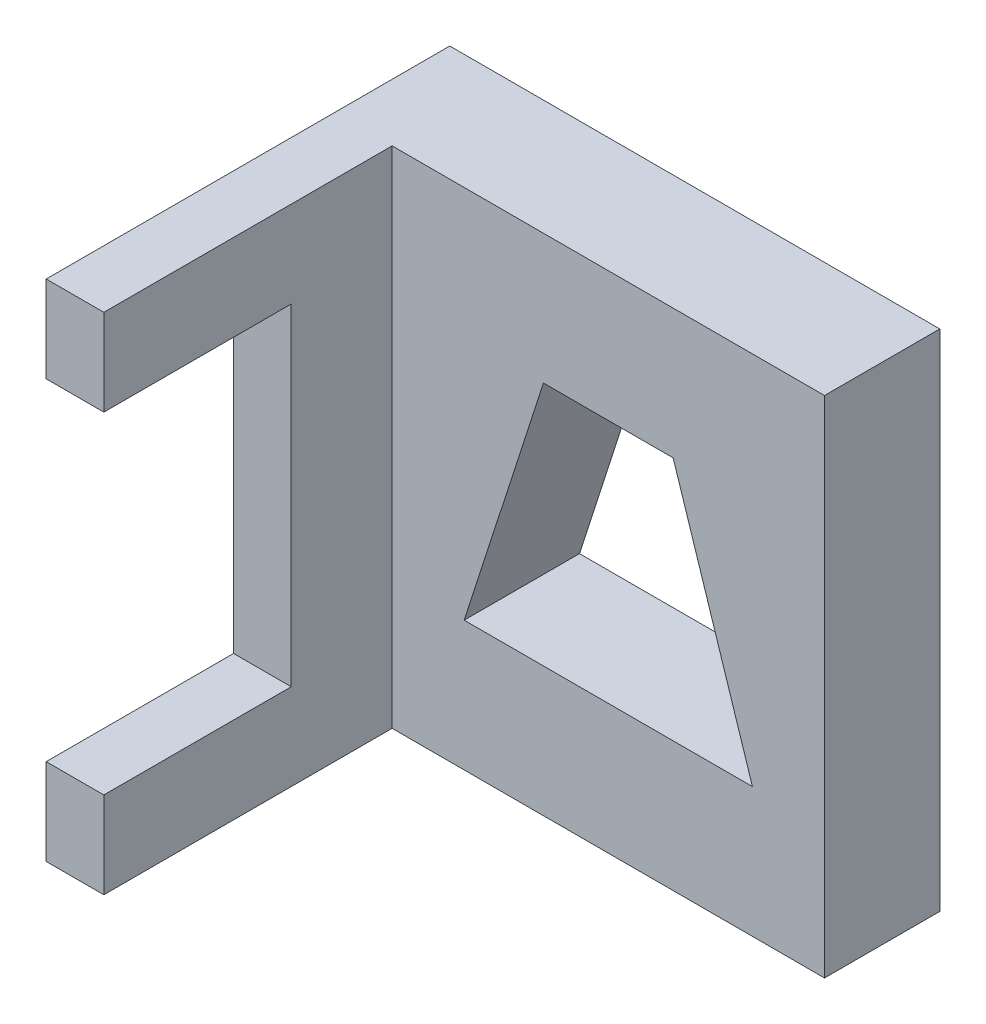
ISO-10303-21;
HEADER;
FILE_DESCRIPTION(('STEP AP214'),'2;1');
FILE_NAME('part.step','',(''),(''),'','','');
FILE_SCHEMA(('AUTOMOTIVE_DESIGN { 1 0 10303 214 1 1 1 1 }'));
ENDSEC;
DATA;
#1=APPLICATION_CONTEXT('core data for automotive mechanical design processes');
#2=APPLICATION_PROTOCOL_DEFINITION('international standard','automotive_design',2000,#1);
#3=PRODUCT_CONTEXT('',#1,'mechanical');
#4=PRODUCT('Part','Part','',(#3));
#5=PRODUCT_RELATED_PRODUCT_CATEGORY('part','',(#4));
#6=PRODUCT_DEFINITION_FORMATION('','',#4);
#7=PRODUCT_DEFINITION_CONTEXT('part definition',#1,'design');
#8=PRODUCT_DEFINITION('design','',#6,#7);
#9=PRODUCT_DEFINITION_SHAPE('','',#8);
#10=(LENGTH_UNIT() NAMED_UNIT(*) SI_UNIT(.MILLI.,.METRE.));
#11=(NAMED_UNIT(*) PLANE_ANGLE_UNIT() SI_UNIT($,.RADIAN.));
#12=(NAMED_UNIT(*) SI_UNIT($,.STERADIAN.) SOLID_ANGLE_UNIT());
#13=UNCERTAINTY_MEASURE_WITH_UNIT(LENGTH_MEASURE(1.E-05),#10,'distance_accuracy_value','');
#14=(GEOMETRIC_REPRESENTATION_CONTEXT(3) GLOBAL_UNCERTAINTY_ASSIGNED_CONTEXT((#13)) GLOBAL_UNIT_ASSIGNED_CONTEXT((#10,
#11,#12)) REPRESENTATION_CONTEXT('',''));
#15=CARTESIAN_POINT('',(0.,0.,0.));
#16=DIRECTION('',(0.,0.,1.));
#17=DIRECTION('',(1.,0.,0.));
#18=AXIS2_PLACEMENT_3D('',#15,#16,#17);
#19=CARTESIAN_POINT('',(0.,0.,16.));
#20=DIRECTION('',(0.,0.,1.));
#21=DIRECTION('',(1.,0.,0.));
#22=AXIS2_PLACEMENT_3D('',#19,#20,#21);
#23=PLANE('',#22);
#24=DIRECTION('',(-0.307820285414663,0.951444518554411,0.));
#25=VECTOR('',#24,1.);
#26=CARTESIAN_POINT('',(47.,52.,16.));
#27=LINE('',#26,#25);
#28=CARTESIAN_POINT('',(58.,18.,16.));
#29=VERTEX_POINT('',#28);
#30=CARTESIAN_POINT('',(47.,52.,16.));
#31=VERTEX_POINT('',#30);
#32=EDGE_CURVE('E58',#29,#31,#27,.T.);
#33=ORIENTED_EDGE('',*,*,#32,.F.);
#34=DIRECTION('',(1.,0.,0.));
#35=VECTOR('',#34,1.);
#36=CARTESIAN_POINT('',(58.,18.,16.));
#37=LINE('',#36,#35);
#38=CARTESIAN_POINT('',(18.,18.,16.));
#39=VERTEX_POINT('',#38);
#40=EDGE_CURVE('E163',#39,#29,#37,.T.);
#41=ORIENTED_EDGE('',*,*,#40,.F.);
#42=DIRECTION('',(-0.307820285414662,-0.951444518554411,0.));
#43=VECTOR('',#42,1.);
#44=CARTESIAN_POINT('',(18.,18.,16.));
#45=LINE('',#44,#43);
#46=CARTESIAN_POINT('',(29.,52.,16.));
#47=VERTEX_POINT('',#46);
#48=EDGE_CURVE('E149',#47,#39,#45,.T.);
#49=ORIENTED_EDGE('',*,*,#48,.F.);
#50=DIRECTION('',(-1.,0.,0.));
#51=VECTOR('',#50,1.);
#52=CARTESIAN_POINT('',(29.,52.,16.));
#53=LINE('',#52,#51);
#54=EDGE_CURVE('E158',#31,#47,#53,.T.);
#55=ORIENTED_EDGE('',*,*,#54,.F.);
#56=EDGE_LOOP('',(#33,#41,#49,#55));
#57=FACE_BOUND('',#56,.T.);
#58=DIRECTION('',(-1.,0.,0.));
#59=VECTOR('',#58,1.);
#60=CARTESIAN_POINT('',(68.,70.,16.));
#61=LINE('',#60,#59);
#62=CARTESIAN_POINT('',(68.,70.,16.));
#63=VERTEX_POINT('',#62);
#64=CARTESIAN_POINT('',(8.,70.,16.));
#65=VERTEX_POINT('',#64);
#66=EDGE_CURVE('E226',#63,#65,#61,.T.);
#67=ORIENTED_EDGE('',*,*,#66,.T.);
#68=DIRECTION('',(0.,-1.,0.));
#69=VECTOR('',#68,1.);
#70=CARTESIAN_POINT('',(8.,0.,16.));
#71=LINE('',#70,#69);
#72=CARTESIAN_POINT('',(8.,0.,16.));
#73=VERTEX_POINT('',#72);
#74=EDGE_CURVE('E215',#65,#73,#71,.T.);
#75=ORIENTED_EDGE('',*,*,#74,.T.);
#76=DIRECTION('',(1.,0.,0.));
#77=VECTOR('',#76,1.);
#78=CARTESIAN_POINT('',(0.,0.,16.));
#79=LINE('',#78,#77);
#80=CARTESIAN_POINT('',(68.,0.,16.));
#81=VERTEX_POINT('',#80);
#82=EDGE_CURVE('E223',#73,#81,#79,.T.);
#83=ORIENTED_EDGE('',*,*,#82,.T.);
#84=DIRECTION('',(0.,1.,0.));
#85=VECTOR('',#84,1.);
#86=CARTESIAN_POINT('',(68.,0.,16.));
#87=LINE('',#86,#85);
#88=EDGE_CURVE('E229',#81,#63,#87,.T.);
#89=ORIENTED_EDGE('',*,*,#88,.T.);
#90=EDGE_LOOP('',(#67,#75,#83,#89));
#91=FACE_BOUND('',#90,.T.);
#92=ADVANCED_FACE('F44',(#57,#91),#23,.T.);
#93=CARTESIAN_POINT('',(0.,70.,16.));
#94=DIRECTION('',(1.,0.,0.));
#95=DIRECTION('',(0.,0.,-1.));
#96=AXIS2_PLACEMENT_3D('',#93,#94,#95);
#97=PLANE('',#96);
#98=DIRECTION('',(0.,-1.,0.));
#99=VECTOR('',#98,1.);
#100=CARTESIAN_POINT('',(0.,70.,0.));
#101=LINE('',#100,#99);
#102=CARTESIAN_POINT('',(0.,70.,0.));
#103=VERTEX_POINT('',#102);
#104=CARTESIAN_POINT('',(0.,0.,0.));
#105=VERTEX_POINT('',#104);
#106=EDGE_CURVE('E221',#103,#105,#101,.T.);
#107=ORIENTED_EDGE('',*,*,#106,.T.);
#108=DIRECTION('',(0.,0.,-1.));
#109=VECTOR('',#108,1.);
#110=CARTESIAN_POINT('',(0.,0.,16.));
#111=LINE('',#110,#109);
#112=CARTESIAN_POINT('',(0.,0.,56.));
#113=VERTEX_POINT('',#112);
#114=EDGE_CURVE('E249',#113,#105,#111,.T.);
#115=ORIENTED_EDGE('',*,*,#114,.F.);
#116=DIRECTION('',(0.,1.,0.));
#117=VECTOR('',#116,1.);
#118=CARTESIAN_POINT('',(0.,0.,56.));
#119=LINE('',#118,#117);
#120=CARTESIAN_POINT('',(0.,12.,56.));
#121=VERTEX_POINT('',#120);
#122=EDGE_CURVE('E173',#113,#121,#119,.T.);
#123=ORIENTED_EDGE('',*,*,#122,.T.);
#124=DIRECTION('',(0.,0.,-1.));
#125=VECTOR('',#124,1.);
#126=CARTESIAN_POINT('',(0.,12.,56.));
#127=LINE('',#126,#125);
#128=CARTESIAN_POINT('',(0.,12.,30.));
#129=VERTEX_POINT('',#128);
#130=EDGE_CURVE('E196',#121,#129,#127,.T.);
#131=ORIENTED_EDGE('',*,*,#130,.T.);
#132=DIRECTION('',(0.,1.,0.));
#133=VECTOR('',#132,1.);
#134=CARTESIAN_POINT('',(0.,12.,30.));
#135=LINE('',#134,#133);
#136=CARTESIAN_POINT('',(0.,58.,30.));
#137=VERTEX_POINT('',#136);
#138=EDGE_CURVE('E203',#129,#137,#135,.T.);
#139=ORIENTED_EDGE('',*,*,#138,.T.);
#140=DIRECTION('',(0.,0.,1.));
#141=VECTOR('',#140,1.);
#142=CARTESIAN_POINT('',(0.,58.,56.));
#143=LINE('',#142,#141);
#144=CARTESIAN_POINT('',(0.,58.,56.));
#145=VERTEX_POINT('',#144);
#146=EDGE_CURVE('E204',#137,#145,#143,.T.);
#147=ORIENTED_EDGE('',*,*,#146,.T.);
#148=DIRECTION('',(0.,1.,0.));
#149=VECTOR('',#148,1.);
#150=CARTESIAN_POINT('',(0.,70.,56.));
#151=LINE('',#150,#149);
#152=CARTESIAN_POINT('',(0.,70.,56.));
#153=VERTEX_POINT('',#152);
#154=EDGE_CURVE('E179',#145,#153,#151,.T.);
#155=ORIENTED_EDGE('',*,*,#154,.T.);
#156=DIRECTION('',(0.,0.,-1.));
#157=VECTOR('',#156,1.);
#158=CARTESIAN_POINT('',(0.,70.,16.));
#159=LINE('',#158,#157);
#160=EDGE_CURVE('E232',#153,#103,#159,.T.);
#161=ORIENTED_EDGE('',*,*,#160,.T.);
#162=EDGE_LOOP('',(#107,#115,#123,#131,#139,#147,#155,#161));
#163=FACE_BOUND('',#162,.T.);
#164=ADVANCED_FACE('F50',(#163),#97,.F.);
#165=CARTESIAN_POINT('',(0.,0.,16.));
#166=DIRECTION('',(0.,1.,0.));
#167=DIRECTION('',(0.,0.,1.));
#168=AXIS2_PLACEMENT_3D('',#165,#166,#167);
#169=PLANE('',#168);
#170=DIRECTION('',(1.,0.,0.));
#171=VECTOR('',#170,1.);
#172=CARTESIAN_POINT('',(0.,0.,0.));
#173=LINE('',#172,#171);
#174=CARTESIAN_POINT('',(68.,0.,0.));
#175=VERTEX_POINT('',#174);
#176=EDGE_CURVE('E235',#105,#175,#173,.T.);
#177=ORIENTED_EDGE('',*,*,#176,.T.);
#178=DIRECTION('',(0.,0.,-1.));
#179=VECTOR('',#178,1.);
#180=CARTESIAN_POINT('',(68.,0.,16.));
#181=LINE('',#180,#179);
#182=EDGE_CURVE('E241',#81,#175,#181,.T.);
#183=ORIENTED_EDGE('',*,*,#182,.F.);
#184=ORIENTED_EDGE('',*,*,#82,.F.);
#185=DIRECTION('',(0.,0.,1.));
#186=VECTOR('',#185,1.);
#187=CARTESIAN_POINT('',(8.,0.,0.));
#188=LINE('',#187,#186);
#189=CARTESIAN_POINT('',(8.,0.,56.));
#190=VERTEX_POINT('',#189);
#191=EDGE_CURVE('E177',#73,#190,#188,.T.);
#192=ORIENTED_EDGE('',*,*,#191,.T.);
#193=DIRECTION('',(-1.,0.,0.));
#194=VECTOR('',#193,1.);
#195=CARTESIAN_POINT('',(8.,0.,56.));
#196=LINE('',#195,#194);
#197=EDGE_CURVE('E195',#190,#113,#196,.T.);
#198=ORIENTED_EDGE('',*,*,#197,.T.);
#199=ORIENTED_EDGE('',*,*,#114,.T.);
#200=EDGE_LOOP('',(#177,#183,#184,#192,#198,#199));
#201=FACE_BOUND('',#200,.T.);
#202=ADVANCED_FACE('F278',(#201),#169,.F.);
#203=CARTESIAN_POINT('',(68.,0.,16.));
#204=DIRECTION('',(-1.,0.,0.));
#205=DIRECTION('',(0.,0.,1.));
#206=AXIS2_PLACEMENT_3D('',#203,#204,#205);
#207=PLANE('',#206);
#208=DIRECTION('',(0.,1.,0.));
#209=VECTOR('',#208,1.);
#210=CARTESIAN_POINT('',(68.,0.,0.));
#211=LINE('',#210,#209);
#212=CARTESIAN_POINT('',(68.,70.,0.));
#213=VERTEX_POINT('',#212);
#214=EDGE_CURVE('E240',#175,#213,#211,.T.);
#215=ORIENTED_EDGE('',*,*,#214,.T.);
#216=DIRECTION('',(0.,0.,-1.));
#217=VECTOR('',#216,1.);
#218=CARTESIAN_POINT('',(68.,70.,16.));
#219=LINE('',#218,#217);
#220=EDGE_CURVE('E244',#63,#213,#219,.T.);
#221=ORIENTED_EDGE('',*,*,#220,.F.);
#222=ORIENTED_EDGE('',*,*,#88,.F.);
#223=ORIENTED_EDGE('',*,*,#182,.T.);
#224=EDGE_LOOP('',(#215,#221,#222,#223));
#225=FACE_BOUND('',#224,.T.);
#226=ADVANCED_FACE('F290',(#225),#207,.F.);
#227=CARTESIAN_POINT('',(68.,70.,16.));
#228=DIRECTION('',(0.,-1.,0.));
#229=DIRECTION('',(0.,0.,-1.));
#230=AXIS2_PLACEMENT_3D('',#227,#228,#229);
#231=PLANE('',#230);
#232=ORIENTED_EDGE('',*,*,#160,.F.);
#233=DIRECTION('',(-1.,0.,0.));
#234=VECTOR('',#233,1.);
#235=CARTESIAN_POINT('',(8.,70.,56.));
#236=LINE('',#235,#234);
#237=CARTESIAN_POINT('',(8.,70.,56.));
#238=VERTEX_POINT('',#237);
#239=EDGE_CURVE('E207',#238,#153,#236,.T.);
#240=ORIENTED_EDGE('',*,*,#239,.F.);
#241=DIRECTION('',(0.,0.,-1.));
#242=VECTOR('',#241,1.);
#243=CARTESIAN_POINT('',(8.,70.,16.));
#244=LINE('',#243,#242);
#245=EDGE_CURVE('E175',#238,#65,#244,.T.);
#246=ORIENTED_EDGE('',*,*,#245,.T.);
#247=ORIENTED_EDGE('',*,*,#66,.F.);
#248=ORIENTED_EDGE('',*,*,#220,.T.);
#249=DIRECTION('',(-1.,0.,0.));
#250=VECTOR('',#249,1.);
#251=CARTESIAN_POINT('',(68.,70.,0.));
#252=LINE('',#251,#250);
#253=EDGE_CURVE('E227',#213,#103,#252,.T.);
#254=ORIENTED_EDGE('',*,*,#253,.T.);
#255=EDGE_LOOP('',(#232,#240,#246,#247,#248,#254));
#256=FACE_BOUND('',#255,.T.);
#257=ADVANCED_FACE('F287',(#256),#231,.F.);
#258=CARTESIAN_POINT('',(0.,0.,0.));
#259=DIRECTION('',(0.,0.,1.));
#260=DIRECTION('',(1.,0.,0.));
#261=AXIS2_PLACEMENT_3D('',#258,#259,#260);
#262=PLANE('',#261);
#263=DIRECTION('',(1.,0.,0.));
#264=VECTOR('',#263,1.);
#265=CARTESIAN_POINT('',(0.,18.,0.));
#266=LINE('',#265,#264);
#267=CARTESIAN_POINT('',(18.,18.,0.));
#268=VERTEX_POINT('',#267);
#269=CARTESIAN_POINT('',(58.,18.,0.));
#270=VERTEX_POINT('',#269);
#271=EDGE_CURVE('E52',#268,#270,#266,.T.);
#272=ORIENTED_EDGE('',*,*,#271,.T.);
#273=DIRECTION('',(-0.307820285414663,0.951444518554411,0.));
#274=VECTOR('',#273,1.);
#275=CARTESIAN_POINT('',(57.7760375880971,18.6922474549726,0.));
#276=LINE('',#275,#274);
#277=CARTESIAN_POINT('',(47.,52.,0.));
#278=VERTEX_POINT('',#277);
#279=EDGE_CURVE('E11',#270,#278,#276,.T.);
#280=ORIENTED_EDGE('',*,*,#279,.T.);
#281=DIRECTION('',(-1.,0.,0.));
#282=VECTOR('',#281,1.);
#283=CARTESIAN_POINT('',(0.,52.,0.));
#284=LINE('',#283,#282);
#285=CARTESIAN_POINT('',(29.,52.,0.));
#286=VERTEX_POINT('',#285);
#287=EDGE_CURVE('E253',#278,#286,#284,.T.);
#288=ORIENTED_EDGE('',*,*,#287,.T.);
#289=DIRECTION('',(-0.307820285414662,-0.951444518554412,0.));
#290=VECTOR('',#289,1.);
#291=CARTESIAN_POINT('',(11.0227094753328,-3.56617071260768,0.));
#292=LINE('',#291,#290);
#293=EDGE_CURVE('E155',#286,#268,#292,.T.);
#294=ORIENTED_EDGE('',*,*,#293,.T.);
#295=EDGE_LOOP('',(#272,#280,#288,#294));
#296=FACE_BOUND('',#295,.T.);
#297=ORIENTED_EDGE('',*,*,#106,.F.);
#298=ORIENTED_EDGE('',*,*,#253,.F.);
#299=ORIENTED_EDGE('',*,*,#214,.F.);
#300=ORIENTED_EDGE('',*,*,#176,.F.);
#301=EDGE_LOOP('',(#297,#298,#299,#300));
#302=FACE_BOUND('',#301,.T.);
#303=ADVANCED_FACE('F254',(#296,#302),#262,.F.);
#304=CARTESIAN_POINT('',(8.,70.,56.));
#305=DIRECTION('',(0.,0.,1.));
#306=DIRECTION('',(1.,0.,0.));
#307=AXIS2_PLACEMENT_3D('',#304,#305,#306);
#308=PLANE('',#307);
#309=ORIENTED_EDGE('',*,*,#154,.F.);
#310=DIRECTION('',(-1.,0.,0.));
#311=VECTOR('',#310,1.);
#312=CARTESIAN_POINT('',(8.,58.,56.));
#313=LINE('',#312,#311);
#314=CARTESIAN_POINT('',(8.,58.,56.));
#315=VERTEX_POINT('',#314);
#316=EDGE_CURVE('E213',#315,#145,#313,.T.);
#317=ORIENTED_EDGE('',*,*,#316,.F.);
#318=DIRECTION('',(0.,1.,0.));
#319=VECTOR('',#318,1.);
#320=CARTESIAN_POINT('',(8.,70.,56.));
#321=LINE('',#320,#319);
#322=EDGE_CURVE('E192',#315,#238,#321,.T.);
#323=ORIENTED_EDGE('',*,*,#322,.T.);
#324=ORIENTED_EDGE('',*,*,#239,.T.);
#325=EDGE_LOOP('',(#309,#317,#323,#324));
#326=FACE_BOUND('',#325,.T.);
#327=ADVANCED_FACE('F286',(#326),#308,.T.);
#328=CARTESIAN_POINT('',(8.,58.,56.));
#329=DIRECTION('',(0.,-1.,0.));
#330=DIRECTION('',(0.,0.,-1.));
#331=AXIS2_PLACEMENT_3D('',#328,#329,#330);
#332=PLANE('',#331);
#333=ORIENTED_EDGE('',*,*,#146,.F.);
#334=DIRECTION('',(-1.,0.,0.));
#335=VECTOR('',#334,1.);
#336=CARTESIAN_POINT('',(8.,58.,30.));
#337=LINE('',#336,#335);
#338=CARTESIAN_POINT('',(8.,58.,30.));
#339=VERTEX_POINT('',#338);
#340=EDGE_CURVE('E214',#339,#137,#337,.T.);
#341=ORIENTED_EDGE('',*,*,#340,.F.);
#342=DIRECTION('',(0.,0.,1.));
#343=VECTOR('',#342,1.);
#344=CARTESIAN_POINT('',(8.,58.,56.));
#345=LINE('',#344,#343);
#346=EDGE_CURVE('E190',#339,#315,#345,.T.);
#347=ORIENTED_EDGE('',*,*,#346,.T.);
#348=ORIENTED_EDGE('',*,*,#316,.T.);
#349=EDGE_LOOP('',(#333,#341,#347,#348));
#350=FACE_BOUND('',#349,.T.);
#351=ADVANCED_FACE('F330',(#350),#332,.T.);
#352=CARTESIAN_POINT('',(8.,12.,30.));
#353=DIRECTION('',(0.,0.,1.));
#354=DIRECTION('',(0.,-1.,0.));
#355=AXIS2_PLACEMENT_3D('',#352,#353,#354);
#356=PLANE('',#355);
#357=ORIENTED_EDGE('',*,*,#138,.F.);
#358=DIRECTION('',(-1.,0.,0.));
#359=VECTOR('',#358,1.);
#360=CARTESIAN_POINT('',(8.,12.,30.));
#361=LINE('',#360,#359);
#362=CARTESIAN_POINT('',(8.,12.,30.));
#363=VERTEX_POINT('',#362);
#364=EDGE_CURVE('E220',#363,#129,#361,.T.);
#365=ORIENTED_EDGE('',*,*,#364,.F.);
#366=DIRECTION('',(0.,1.,0.));
#367=VECTOR('',#366,1.);
#368=CARTESIAN_POINT('',(8.,12.,30.));
#369=LINE('',#368,#367);
#370=EDGE_CURVE('E188',#363,#339,#369,.T.);
#371=ORIENTED_EDGE('',*,*,#370,.T.);
#372=ORIENTED_EDGE('',*,*,#340,.T.);
#373=EDGE_LOOP('',(#357,#365,#371,#372));
#374=FACE_BOUND('',#373,.T.);
#375=ADVANCED_FACE('F324',(#374),#356,.T.);
#376=CARTESIAN_POINT('',(8.,12.,56.));
#377=DIRECTION('',(0.,1.,0.));
#378=DIRECTION('',(0.,0.,1.));
#379=AXIS2_PLACEMENT_3D('',#376,#377,#378);
#380=PLANE('',#379);
#381=ORIENTED_EDGE('',*,*,#130,.F.);
#382=DIRECTION('',(-1.,0.,0.));
#383=VECTOR('',#382,1.);
#384=CARTESIAN_POINT('',(8.,12.,56.));
#385=LINE('',#384,#383);
#386=CARTESIAN_POINT('',(8.,12.,56.));
#387=VERTEX_POINT('',#386);
#388=EDGE_CURVE('E218',#387,#121,#385,.T.);
#389=ORIENTED_EDGE('',*,*,#388,.F.);
#390=DIRECTION('',(0.,0.,-1.));
#391=VECTOR('',#390,1.);
#392=CARTESIAN_POINT('',(8.,12.,56.));
#393=LINE('',#392,#391);
#394=EDGE_CURVE('E181',#387,#363,#393,.T.);
#395=ORIENTED_EDGE('',*,*,#394,.T.);
#396=ORIENTED_EDGE('',*,*,#364,.T.);
#397=EDGE_LOOP('',(#381,#389,#395,#396));
#398=FACE_BOUND('',#397,.T.);
#399=ADVANCED_FACE('F325',(#398),#380,.T.);
#400=CARTESIAN_POINT('',(8.,0.,56.));
#401=DIRECTION('',(0.,0.,1.));
#402=DIRECTION('',(1.,0.,0.));
#403=AXIS2_PLACEMENT_3D('',#400,#401,#402);
#404=PLANE('',#403);
#405=ORIENTED_EDGE('',*,*,#122,.F.);
#406=ORIENTED_EDGE('',*,*,#197,.F.);
#407=DIRECTION('',(0.,1.,0.));
#408=VECTOR('',#407,1.);
#409=CARTESIAN_POINT('',(8.,0.,56.));
#410=LINE('',#409,#408);
#411=EDGE_CURVE('E180',#190,#387,#410,.T.);
#412=ORIENTED_EDGE('',*,*,#411,.T.);
#413=ORIENTED_EDGE('',*,*,#388,.T.);
#414=EDGE_LOOP('',(#405,#406,#412,#413));
#415=FACE_BOUND('',#414,.T.);
#416=ADVANCED_FACE('F269',(#415),#404,.T.);
#417=CARTESIAN_POINT('',(8.,0.,0.));
#418=DIRECTION('',(-1.,0.,0.));
#419=DIRECTION('',(0.,0.,1.));
#420=AXIS2_PLACEMENT_3D('',#417,#418,#419);
#421=PLANE('',#420);
#422=ORIENTED_EDGE('',*,*,#74,.F.);
#423=ORIENTED_EDGE('',*,*,#245,.F.);
#424=ORIENTED_EDGE('',*,*,#322,.F.);
#425=ORIENTED_EDGE('',*,*,#346,.F.);
#426=ORIENTED_EDGE('',*,*,#370,.F.);
#427=ORIENTED_EDGE('',*,*,#394,.F.);
#428=ORIENTED_EDGE('',*,*,#411,.F.);
#429=ORIENTED_EDGE('',*,*,#191,.F.);
#430=EDGE_LOOP('',(#422,#423,#424,#425,#426,#427,#428,#429));
#431=FACE_BOUND('',#430,.T.);
#432=ADVANCED_FACE('F265',(#431),#421,.F.);
#433=CARTESIAN_POINT('',(47.,52.,-2.));
#434=DIRECTION('',(0.951444518554411,0.307820285414662,0.));
#435=DIRECTION('',(-0.307820285414663,0.951444518554411,0.));
#436=AXIS2_PLACEMENT_3D('',#433,#434,#435);
#437=PLANE('',#436);
#438=DIRECTION('',(0.,0.,1.));
#439=VECTOR('',#438,1.);
#440=CARTESIAN_POINT('',(58.,18.,-2.));
#441=LINE('',#440,#439);
#442=EDGE_CURVE('E166',#270,#29,#441,.T.);
#443=ORIENTED_EDGE('',*,*,#442,.T.);
#444=ORIENTED_EDGE('',*,*,#32,.T.);
#445=DIRECTION('',(0.,0.,1.));
#446=VECTOR('',#445,1.);
#447=CARTESIAN_POINT('',(47.,52.,-2.));
#448=LINE('',#447,#446);
#449=EDGE_CURVE('E154',#278,#31,#448,.T.);
#450=ORIENTED_EDGE('',*,*,#449,.F.);
#451=ORIENTED_EDGE('',*,*,#279,.F.);
#452=EDGE_LOOP('',(#443,#444,#450,#451));
#453=FACE_BOUND('',#452,.T.);
#454=ADVANCED_FACE('F257',(#453),#437,.F.);
#455=CARTESIAN_POINT('',(58.,18.,-2.));
#456=DIRECTION('',(0.,-1.,0.));
#457=DIRECTION('',(0.,0.,-1.));
#458=AXIS2_PLACEMENT_3D('',#455,#456,#457);
#459=PLANE('',#458);
#460=DIRECTION('',(0.,0.,1.));
#461=VECTOR('',#460,1.);
#462=CARTESIAN_POINT('',(18.,18.,-2.));
#463=LINE('',#462,#461);
#464=EDGE_CURVE('E152',#268,#39,#463,.T.);
#465=ORIENTED_EDGE('',*,*,#464,.T.);
#466=ORIENTED_EDGE('',*,*,#40,.T.);
#467=ORIENTED_EDGE('',*,*,#442,.F.);
#468=ORIENTED_EDGE('',*,*,#271,.F.);
#469=EDGE_LOOP('',(#465,#466,#467,#468));
#470=FACE_BOUND('',#469,.T.);
#471=ADVANCED_FACE('F259',(#470),#459,.F.);
#472=CARTESIAN_POINT('',(18.,18.,-2.));
#473=DIRECTION('',(-0.951444518554411,0.307820285414662,0.));
#474=DIRECTION('',(-0.307820285414662,-0.951444518554412,0.));
#475=AXIS2_PLACEMENT_3D('',#472,#473,#474);
#476=PLANE('',#475);
#477=DIRECTION('',(0.,0.,1.));
#478=VECTOR('',#477,1.);
#479=CARTESIAN_POINT('',(29.,52.,-2.));
#480=LINE('',#479,#478);
#481=EDGE_CURVE('E69',#286,#47,#480,.T.);
#482=ORIENTED_EDGE('',*,*,#481,.T.);
#483=ORIENTED_EDGE('',*,*,#48,.T.);
#484=ORIENTED_EDGE('',*,*,#464,.F.);
#485=ORIENTED_EDGE('',*,*,#293,.F.);
#486=EDGE_LOOP('',(#482,#483,#484,#485));
#487=FACE_BOUND('',#486,.T.);
#488=ADVANCED_FACE('F148',(#487),#476,.F.);
#489=CARTESIAN_POINT('',(29.,52.,-2.));
#490=DIRECTION('',(0.,1.,0.));
#491=DIRECTION('',(0.,0.,1.));
#492=AXIS2_PLACEMENT_3D('',#489,#490,#491);
#493=PLANE('',#492);
#494=ORIENTED_EDGE('',*,*,#449,.T.);
#495=ORIENTED_EDGE('',*,*,#54,.T.);
#496=ORIENTED_EDGE('',*,*,#481,.F.);
#497=ORIENTED_EDGE('',*,*,#287,.F.);
#498=EDGE_LOOP('',(#494,#495,#496,#497));
#499=FACE_BOUND('',#498,.T.);
#500=ADVANCED_FACE('F157',(#499),#493,.F.);
#501=CLOSED_SHELL('',(#92,#164,#202,#226,#257,#303,#327,#351,#375,#399,#416,#432,#454,#471,#488,#500));
#502=MANIFOLD_SOLID_BREP('B2',#501);
#503=ADVANCED_BREP_SHAPE_REPRESENTATION('',(#18,#502),#14);
#504=SHAPE_DEFINITION_REPRESENTATION(#9,#503);
ENDSEC;
END-ISO-10303-21;
